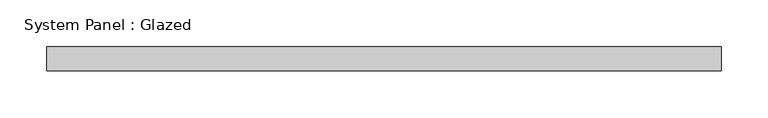
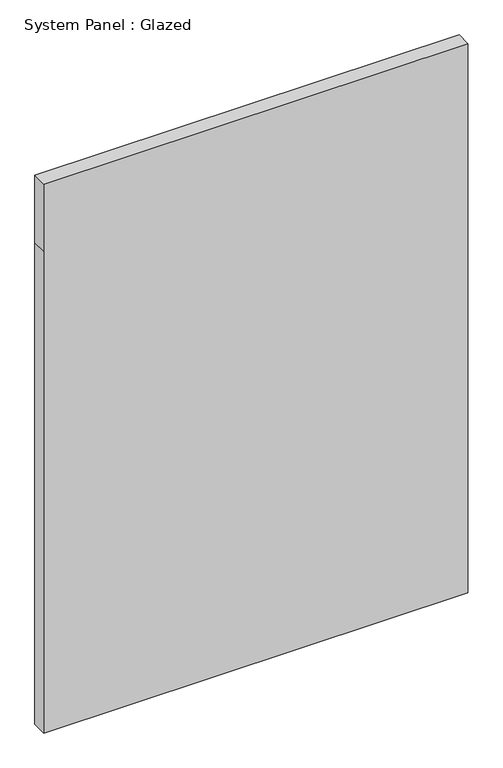
"""IFC4 building model written with IfcOpenShell, lengths in millimetres: plate geometry, System Panel : Glazed."""

from ifc_helpers import new_model, si_unit, frame, origin, place, context, project, spatial, polyline, outline, extrude, source, transform, mapped, element, save


def system_panel_glazed_52336633(model_context):
    return source(origin(), model_context, "Body", "SweptSolid", [
        extrude(outline(polyline([(0.0, -358.775), (0.0, 358.775), (861.2594531, 358.775), (981.9094531, 358.775), (981.9094531, -358.775), (861.2594531, -358.775), (0.0, -358.775)])), frame((0.0, 19.05, 0.0), z_axis=(0.0, 1.0, 0.0), x_axis=(0.0, 0.0, 1.0)), (0.0, 0.0, 1.0), 25.4),
    ])


if __name__ == "__main__":
    model = new_model("IFC4")
    model_context = context("Model", 3, world=origin())
    ifc_project = project(units=[si_unit("LENGTHUNIT", "METRE", prefix="MILLI")], contexts=[model_context])
    site = spatial("IfcSite", under=ifc_project)
    building = spatial("IfcBuilding", under=site)
    placement = place(None, origin())
    system_panel_glazed_shape = system_panel_glazed_52336633(model_context)
    element("IfcPlate", 1, ObjectType="System Panel : Glazed", at=placement, inside=building, context=model_context, shape_type="MappedRepresentation", body=[
        mapped(system_panel_glazed_shape, transform((0.0, 0.0, 0.0), x_axis=(1.0, 0.0, 0.0), y_axis=(0.0, 1.0, 0.0), z_axis=(0.0, 0.0, 1.0))),
    ])
    save(model, "model.ifc")

# Revit data of these elements
# Type "System Panel : Glazed"
#   Construction Type Id = "GSP4R"
#   Analytic Construction = "1/8 in Pilkington single glazing"
#   Visual Light Transmittance = 0.9
#   Solar Heat Gain Coefficient = 0.86
#   Heat Transfer Coefficient (U) = 1.18115 BTU/(h·ft²·°F)
#   Define Thermal Properties by = 1
# Element 1 (IfcPlate, "System Panel : Glazed")
#   Materials on its faces: "Glass"
# Materials
#   "Glass": class "Glass", colour RGB 0 128 192, transparency 0.75, Description = "Soda Lime Glass", Cost = 0
